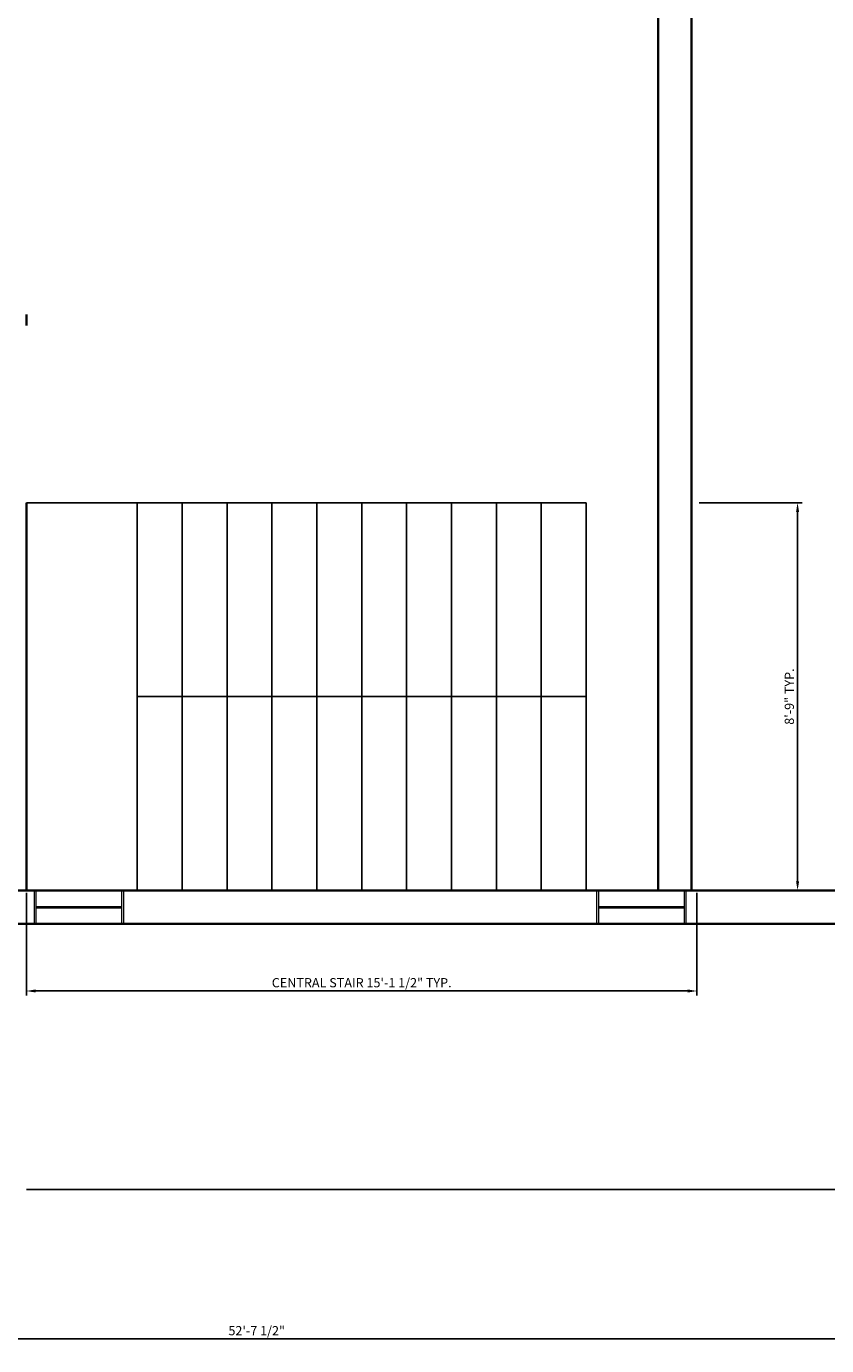
# Model space of a CAD drawing. Units: inches. Extents: x 250205121 to 250208111, y 89832590 to 89833271.
# Tile 11 of 14: x 250207593 to 250207809, y 89832598 to 89832955. Entities that reach past the tile are written whole.
import ezdxf

# ---------------------------------------------------------------- set-up
doc = ezdxf.new("R2010")
doc.units = ezdxf.units.IN
for name, color, linetype, lineweight in [('A-FLOR-STRS', 7, 'Continuous', 25), ('A-WALL', 7, 'Continuous', 35), ('C-PROP', 8, 'Continuous', 25), ('dimensions', 2, 'Continuous', 18), ('window', 4, 'Continuous', 18)]:
    doc.layers.add(name, color=color, linetype=linetype, lineweight=lineweight)
doc.styles.get("Standard").update_dxf_attribs({"font": 'arial.ttf'})
doc.dimstyles.new('ISO-25', dxfattribs={"dimtxt": 2.5, "dimasz": 2.5, "dimexe": 1.25, "dimexo": 0.625, "dimtad": 1, "dimlunit": 4, "dimtxsty": 'Standard', "dimcen": 2.5, "dimadec": 0, "dimazin": 0, "dimtfac": 1, "dimtmove": 0, "dimatfit": 3, "dimfxl": 1, "dimarcsym": 0})

# ---------------------------------------------------------------- blocks, each defined once
blk = doc.blocks.new('WIN-24IN')
for p, q in [((0, 0), (0, 24.08)), ((0, 24.08), (9, 24.08)), ((0, 23.58), (9, 23.58)), ((4.3, 23.58), (4.3, 0.5)), ((4.7, 23.58), (4.7, 0.5)), ((9, 24.08), (9, 0)), ((9, 0.5), (0, 0.5)), ((9, 0), (0, 0))]:
    blk.add_line(p, q)
blk = doc.blocks.new('STAIR-CENTRAL')
for p, q in [((0, 105), (30, 105)), ((30, 105), (30, 0)), ((30, 105), (151.5, 105)), ((42.15, 105), (42.15, 0)), ((54.3, 105), (54.3, 0)), ((66.45, 105), (66.45, 0)), ((78.6, 105), (78.6, 0)), ((90.75, 105), (90.75, 0)), ((102.9, 105), (102.9, 0)), ((115.05, 105), (115.05, 0)), ((127.2, 105), (127.2, 0)), ((139.35, 105), (139.35, 0)), ((151.5, 105), (151.5, 0)), ((151.5, 105), (151.5, 0)), ((151.5, 52.5), (30, 52.5)), ((0, 0), (6, 0)), ((6, 0), (30, 0)), ((30, 0), (151.5, 0)), ((151.5, 0), (175.5, 0)), ((175.5, 0), (181.5, 0))]:
    blk.add_line(p, q)
blk = doc.blocks.new('*D39')
at = {"layer": 'Defpoints', "color": 0, "transparency": 16777216}
for p in [(250207592.71, 89832721.22), (250207774.21, 89832721.22), (250207774.21, 89832693.99)]:
    blk.add_point(p, dxfattribs=at)
at = {"layer": 'dimensions', "color": 0, "lineweight": -2, "transparency": 16777216}
for p, q in [((250207592.71, 89832720.59), (250207592.71, 89832692.74)), ((250207774.21, 89832720.59), (250207774.21, 89832692.74)), ((250207595.21, 89832693.99), (250207771.71, 89832693.99))]:
    blk.add_line(p, q, dxfattribs=at)
at = {"layer": 'dimensions', "color": 0, "transparency": 16777216}
for points in [[(250207595.21, 89832694.41), (250207595.21, 89832693.58), (250207592.71, 89832693.99)], [(250207771.71, 89832694.41), (250207771.71, 89832693.58), (250207774.21, 89832693.99)]]:
    blk.add_solid(points, dxfattribs=at)
at = {"layer": 'dimensions', "color": 0, "transparency": 16777216, "insert": (250207683.46, 89832695.91), "char_height": 2.5, "attachment_point": 5}
blk.add_mtext('CENTRAL STAIR 15\'-1 1/2" TYP.', dxfattribs=at)
blk = doc.blocks.new('*D40')
at = {"layer": 'Defpoints', "color": 0, "transparency": 16777216}
for p in [(250207774.21, 89832826.22), (250207801.43, 89832826.22), (250207774.21, 89832721.22)]:
    blk.add_point(p, dxfattribs=at)
at = {"layer": 'dimensions', "color": 0, "lineweight": -2, "transparency": 16777216}
for p, q in [((250207774.83, 89832826.22), (250207802.68, 89832826.22)), ((250207801.43, 89832723.72), (250207801.43, 89832823.72)), ((250207774.83, 89832721.22), (250207802.68, 89832721.22))]:
    blk.add_line(p, q, dxfattribs=at)
at = {"layer": 'dimensions', "color": 0, "transparency": 16777216}
for points in [[(250207801.02, 89832823.72), (250207801.85, 89832823.72), (250207801.43, 89832826.22)], [(250207801.02, 89832723.72), (250207801.85, 89832723.72), (250207801.43, 89832721.22)]]:
    blk.add_solid(points, dxfattribs=at)
at = {"layer": 'dimensions', "color": 0, "transparency": 16777216, "insert": (250207799.53, 89832773.72), "char_height": 2.5, "attachment_point": 5, "rotation": 90}
blk.add_mtext('8\'-9" TYP.', dxfattribs=at)
blk = doc.blocks.new('*D70')
at = {"layer": 'Defpoints', "color": 0, "transparency": 16777216}
for p in [(250207339.21, 89832712.22), (250207970.87, 89832712.22), (250207970.87, 89832599.77)]:
    blk.add_point(p, dxfattribs=at)
at = {"layer": 'dimensions', "color": 0, "lineweight": -2, "transparency": 16777216}
for p, q in [((250207339.21, 89832711.59), (250207339.21, 89832598.52)), ((250207970.87, 89832711.59), (250207970.87, 89832598.52)), ((250207341.71, 89832599.77), (250207968.37, 89832599.77))]:
    blk.add_line(p, q, dxfattribs=at)
at = {"layer": 'dimensions', "color": 0, "transparency": 16777216}
for points in [[(250207341.71, 89832600.18), (250207341.71, 89832599.35), (250207339.21, 89832599.77)], [(250207968.37, 89832600.18), (250207968.37, 89832599.35), (250207970.87, 89832599.77)]]:
    blk.add_solid(points, dxfattribs=at)
at = {"layer": 'dimensions', "color": 0, "transparency": 16777216, "insert": (250207655.04, 89832601.68), "char_height": 2.5, "attachment_point": 5}
blk.add_mtext('52\'-7 1/2"', dxfattribs=at)

msp = doc.modelspace()

# ---------------------------------------------------------------- linework, layer by layer
at = {"layer": 'A-WALL'}
for p, q in [((250207763.707, 89832721.217), (250207763.707, 89833132.217)), ((250207772.707, 89832721.217), (250207772.707, 89833132.217)), ((250207592.707, 89832877.217), (250207592.707, 89832874.217)), ((250207592.707, 89832826.217), (250207592.707, 89832721.217)), ((250207889.707, 89832721.217), (250207348.207, 89832721.217)), ((250207889.707, 89832712.217), (250207356.707, 89832712.217))]:
    msp.add_line(p, q, dxfattribs=at)
at = {"layer": 'C-PROP'}
msp.add_line((250208069.707, 89832640.217), (250207592.707, 89832640.217), dxfattribs=at)

# ---------------------------------------------------------------- block references
at = {"layer": 'A-FLOR-STRS'}
msp.add_blockref('STAIR-CENTRAL', (250207592.707, 89832721.217), dxfattribs=at)
at = {"layer": 'window'}
for p, rotation in [((250207618.957, 89832712.217), 90.00000018666607), ((250207771.207, 89832712.217), 90.00000024888803)]:
    msp.add_blockref('WIN-24IN', p, dxfattribs=dict(at, rotation=rotation))

# ---------------------------------------------------------------- dimensions: what is measured, and where the dimension line sits
at = {"layer": 'dimensions'}
dim = msp.add_linear_dim(base=(250207801.432, 89832826.217), p1=(250207774.207, 89832721.217), p2=(250207774.207, 89832826.217), angle=90, text='<> TYP.', dimstyle='ISO-25', override={"dimdec": 1, "dimlfac": 1, "dimrnd": 0, "dimzin": 1, "dimdsep": 46, "dimlunit": 4, "dimfrac": 2}, dxfattribs=at)
dim.commit()
dim.dimension.update_dxf_attribs({"geometry": '*D40', "text_midpoint": (250207799.531, 89832773.717)})
dim = msp.add_linear_dim(base=(250207774.207, 89832693.992), p1=(250207592.707, 89832721.217), p2=(250207774.207, 89832721.217), text='CENTRAL STAIR <> TYP.', dimstyle='ISO-25', override={"dimdec": 1, "dimlfac": 1, "dimrnd": 0, "dimzin": 1, "dimdsep": 46, "dimlunit": 4, "dimfrac": 2}, dxfattribs=at)
dim.commit()
dim.dimension.update_dxf_attribs({"geometry": '*D39', "text_midpoint": (250207683.457, 89832695.91)})
dim = msp.add_linear_dim(base=(250207970.867, 89832599.767), p1=(250207339.207, 89832712.217), p2=(250207970.867, 89832712.217), dimstyle='ISO-25', override={"dimdec": 1, "dimlfac": 1, "dimrnd": 0, "dimzin": 1, "dimdsep": 46, "dimlunit": 4, "dimfrac": 2}, dxfattribs=at)
dim.commit()
dim.dimension.update_dxf_attribs({"geometry": '*D70', "text_midpoint": (250207655.037, 89832601.685)})

doc.saveas('drawing.dxf')
